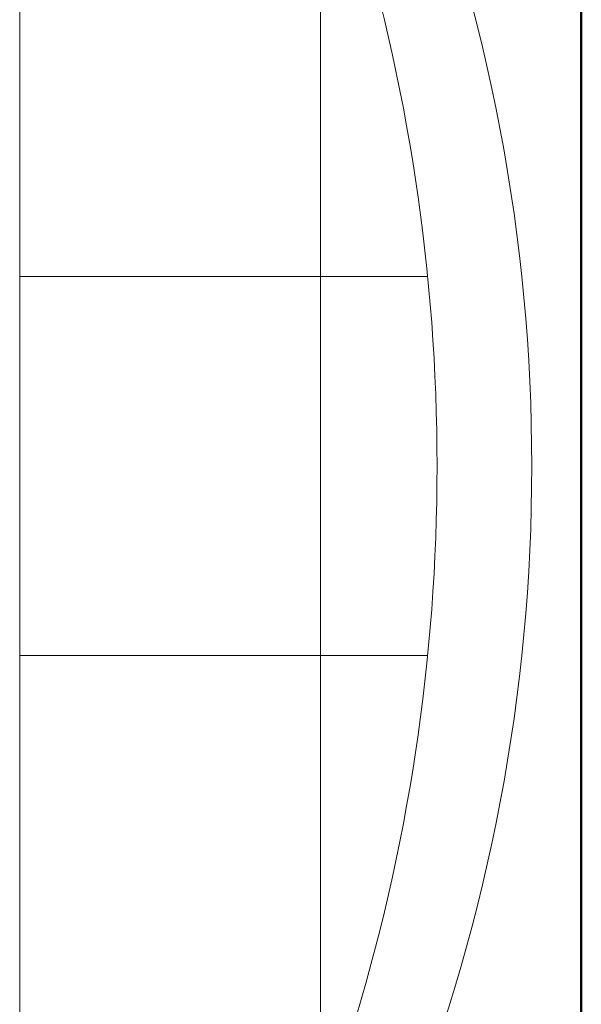
# Model space of a CAD drawing. Units: inches. Extents: x -105 to 1196, y -792 to 119.
# Tile 15 of 23: x 279 to 315, y -380 to -318. Entities that reach past the tile are written whole.
import ezdxf

# ---------------------------------------------------------------- set-up
doc = ezdxf.new("R2010")
doc.units = ezdxf.units.IN
doc.header["$MEASUREMENT"] = 0
doc.layers.add('A-FURN', color=8, linetype='Continuous', lineweight=18)
doc.layers.add('A-WALL', color=3, linetype='Continuous', lineweight=50)

# ---------------------------------------------------------------- blocks, each defined once
blk = doc.blocks.new('Sofa - Roundback 7 ft.')
for p, q in [((-12.00002, -32.4421), (-12.00003, -6.5971)), ((11.99997, -32.4421), (11.99998, -6.5971)), ((-35.999844, -13.3819), (35.9998, -13.3819)), ((-36.000027, -32.4421), (35.99998, -32.4421))]:
    blk.add_line(p, q)
for centre, radius, start, end in [((0, -114.25), 114.25, 68.43141, 111.5686), ((-0.00001, -127.1968), 121.1968, 72.72033, 107.2797)]:
    blk.add_arc(centre, radius, start, end)

msp = doc.modelspace()

# ---------------------------------------------------------------- linework, layer by layer
at = {"layer": 'A-WALL'}
msp.add_line((314.744, -268.115), (314.744, -429.227), dxfattribs=at)

# ---------------------------------------------------------------- block references
at = {"layer": 'A-FURN', "rotation": 270}
msp.add_blockref('Sofa - Roundback 7 ft.', (311.607, -346.122), dxfattribs=at)

doc.saveas('drawing.dxf')
